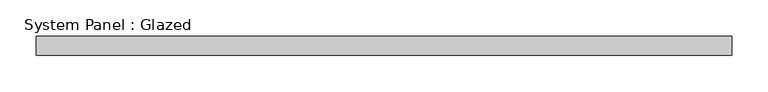
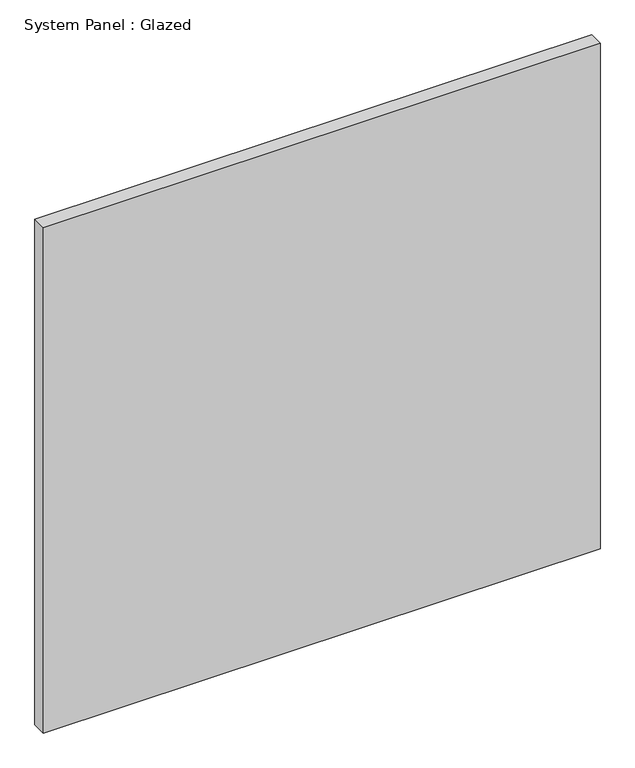
"""IFC4 building model written with IfcOpenShell, lengths in millimetres: plate geometry, System Panel : Glazed."""

from ifc_helpers import new_model, si_unit, origin, origin_with_axes, place, context, project, spatial, polyline, outline, extrude, source, transform, mapped, element, save


def system_panel_glazed_1eaf0385(model_context):
    return source(origin(), model_context, "Body", "SweptSolid", [
        extrude(outline(polyline([(476.3180043, 19.05), (-476.3180043, 19.05), (-476.3180043, 44.45), (476.3180043, 44.45), (476.3180043, 19.05)])), origin_with_axes(), (0.0, 0.0, 1.0), 914.4),
    ])


if __name__ == "__main__":
    model = new_model("IFC4")
    model_context = context("Model", 3, world=origin())
    ifc_project = project(units=[si_unit("LENGTHUNIT", "METRE", prefix="MILLI")], contexts=[model_context])
    site = spatial("IfcSite", under=ifc_project)
    building = spatial("IfcBuilding", under=site)
    placement = place(None, origin())
    system_panel_glazed_shape = system_panel_glazed_1eaf0385(model_context)
    element("IfcPlate", 1, ObjectType="System Panel : Glazed", at=placement, inside=building, context=model_context, shape_type="MappedRepresentation", body=[
        mapped(system_panel_glazed_shape, transform((0.0, 0.0, 0.0), x_axis=(1.0, 0.0, 0.0), y_axis=(0.0, 1.0, 0.0), z_axis=(0.0, 0.0, 1.0))),
    ])
    save(model, "model.ifc")

# Revit data of these elements
# Type "System Panel : Glazed"
#   Construction Type Id = "GSP4R"
#   Analytic Construction = "1/8 in Pilkington single glazing"
#   Visual Light Transmittance = 0.9
#   Solar Heat Gain Coefficient = 0.86
#   Heat Transfer Coefficient (U) = 1.18115 BTU/(h·ft²·°F)
# Element 1 (IfcPlate, "System Panel : Glazed")
#   Materials on its faces: "Glass"
# Materials
#   "Glass": class "Glass", colour RGB 0 128 192, transparency 0.75, Description = "Soda Lime Glass", Cost = 0
